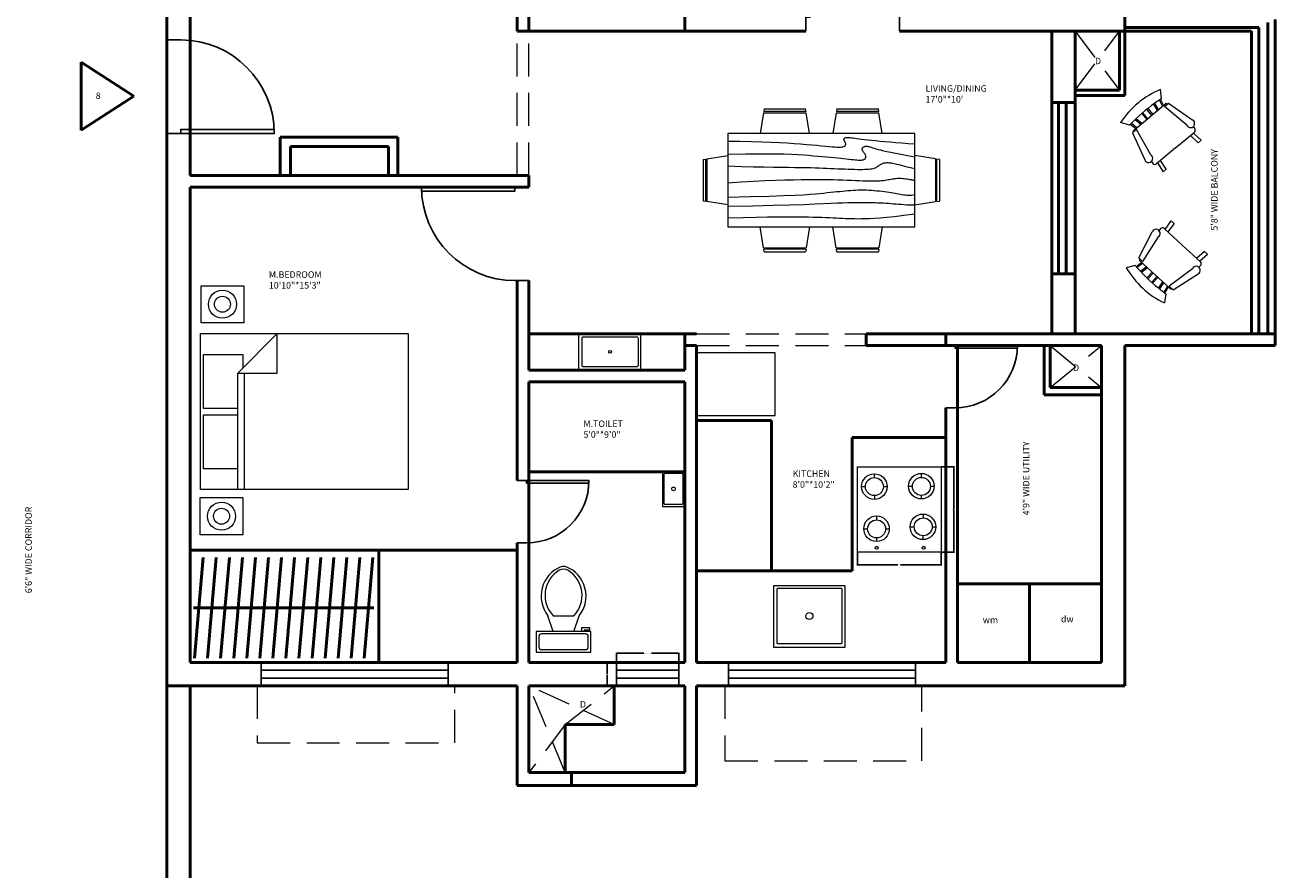
# Model space of a CAD drawing. Units: inches. Extents: x 291 to 2631, y 456 to 2623.
# Tile 12 of 22: x 2114 to 2595, y 1042 to 1367. Entities that reach past the tile are written whole.
import ezdxf

# ---------------------------------------------------------------- set-up
doc = ezdxf.new("R2010")
doc.units = ezdxf.units.IN
doc.linetypes.add('DASHED', pattern=[19.05, 12.7, -6.35])
for name, color, linetype, lineweight in [('A-ANNO-DIMS', 2, 'Continuous', 18), ('A-ANNO-TEXT', 3, 'Continuous', 25), ('A-AREA-IDEN', 7, 'Continuous', 25), ('A-DOOR', 3, 'Continuous', 25), ('A-EQPM', 8, 'Continuous', 18), ('A-FLOR-FIXT', 9, 'Continuous', 18), ('A-FLOR-OVHD', 1, 'DASHED', 18), ('A-FURN', 8, 'Continuous', 18), ('A-GLAZ', 4, 'Continuous', 25), ('A-WALL', 7, 'Continuous', 50)]:
    doc.layers.add(name, color=color, linetype=linetype, lineweight=lineweight)
doc.styles.get("Standard").update_dxf_attribs({"font": 'arial.ttf'})
doc.dimstyles.get("Standard").update_dxf_attribs({"dimtxt": 0.18, "dimasz": 0.18, "dimexe": 0.18, "dimexo": 0.0625, "dimgap": 0.09, "dimtad": 0, "dimtih": 1, "dimtoh": 1, "dimdec": 4, "dimzin": 0, "dimdsep": 46, "dimtxsty": 'Standard', "dimcen": 0.09, "dimadec": 0, "dimazin": 0, "dimtfac": 1, "dimtdec": 4, "dimtofl": 0, "dimtmove": 0, "dimatfit": 3, "dimfxl": 1, "dimtolj": 1, "dimtzin": 0, "dimarcsym": 0})

# ---------------------------------------------------------------- blocks, each defined once
blk = doc.blocks.new('*U2')
for p, q in [((0, 0), (0, -6)), ((40, 0), (40, -6))]:
    blk.add_line(p, q)
blk.add_lwpolyline([(0, 0), (0, 40), (1.75, 40), (1.75, 0)], close=True)
blk.add_arc((0, 0), 40, 0, 90)
blk = doc.blocks.new('Bed - Queen')
for p, q in [((0, -80.00003), (0, 0)), ((0, 0), (59.99999, 0)), ((59.99999, 0), (59.99999, -80.00003)), ((7.99999, -1.2), (28.79998, -1.2)), ((7.99999, -14.4), (7.99999, -1.2)), ((28.79998, -1.2), (28.79998, -14.4)), ((31.19999, -1.2), (51.99999, -1.2)), ((31.19999, -14.4), (31.19999, -1.2)), ((51.99999, -1.2), (51.99999, -16.4)), ((0, -14.4), (44.8, -14.4)), ((59.99999, -29.6), (44.8, -14.4)), ((44.8, -14.4), (44.8, -29.6)), ((44.8, -16.8), (0, -16.8)), ((51.99999, -16.4), (46.79936, -16.4)), ((44.8, -29.6), (59.99999, -29.6)), ((59.99999, -80.00003), (0, -80.00003))]:
    blk.add_line(p, q)
blk = doc.blocks.new('Toilet - top')
for p, q in [((9.5, -6), (9.5, -2)), ((-10, -8.5), (-8, -8.5)), ((-10, -9.5), (-10, -8.5)), ((-7, -9.5), (-10, -9.5)), ((-8, -8.5), (-8, -8)), ((-7, -8), (-7, -9.5)), ((-4, -8), (-6, -14)), ((4, -8), (6, -14)), ((4, -14), (-4, -14))]:
    blk.add_line(p, q)
blk.add_lwpolyline([(10.5, -8), (10.5, 0), (-10.5, 0), (-10.5, -8)], close=True)
for points in [[(-9.5, -2), (-9.5, -6)], [(8.5, -1), (-8.5, -1)], [(-8.5, -7), (8.5, -7)]]:
    blk.add_lwpolyline(points)
for centre, radius, start, end in [((-8.62, -1.88), 0.884, 81.8699, 188.1301), ((8.62, -1.88), 0.884, 351.8699, 98.1301), ((-8.62, -6.12), 0.884, 171.8699, 278.1301), ((8.62, -6.12), 0.884, 261.8699, 8.1301), ((3.52, -21.58), 12.17, 141.4691, 247.9714), ((4.2, -21.82), 11.33, 136.3677, 238.9468), ((-3.52, -21.58), 12.17, 292.0284, 38.5307), ((-4.2, -21.82), 11.33, 301.053, 43.6321), ((0, -27.88), 4, 245.7318, 294.2682), ((0, -29), 4, 254.8605, 285.1395)]:
    blk.add_arc(centre, radius, start, end)
blk = doc.blocks.new('Chair - Rocking')
for p, q in [((-8, -4.5), (-10, -1.5)), ((-7.5, -4.5), (-7, -7)), ((-6.5, -7), (-7.02225, -4.43)), ((-4.5, -7), (-4.96674, -4.19951)), ((-4, -7), (-4.40532, -4.16272)), ((-1.5, -4.05012), (-1.5, -7)), ((-1, -7), (-1, -4.05012)), ((1, -7), (1, -4.04655)), ((1.5, -4.05012), (1.5, -7)), ((4, -7), (4.40187, -4.18694)), ((4.5, -7), (4.96761, -4.19437)), ((6.5, -7), (7, -4.4057)), ((7.5, -4.5), (7, -7)), ((8, -4.5), (10, -1.5)), ((-9, -7.5), (-12, -18.49999)), ((-7, -7.5), (-9, -7.5)), ((-9, -18.49999), (-7, -7.5)), ((-8.23428, -6.99939), (-8.3093, -7.47958)), ((-8.23041, -7), (8.23915, -7)), ((7, -7.5), (9, -7.5)), ((9, -18.49999), (7, -7.5)), ((8.31071, -7.48854), (8.23449, -7.00073)), ((9, -7.5), (12, -18.49999)), ((-10.36644, -20.64523), (-10.5, -21.49999)), ((-9, -22.49999), (-9.5, -26.49999)), ((0, -22.49999), (-9.5, -22.49999)), ((-8, -26.49999), (-7.5, -22.49999)), ((0, -22.49999), (9.5, -22.49999)), ((8, -26.49999), (7.5, -22.49999)), ((9, -22.49999), (9.5, -26.49999)), ((10.5, -21.49999), (10.3575, -20.58798)), ((-9.5, -26.49999), (-8, -26.49999)), ((9.5, -26.49999), (8, -26.49999))]:
    blk.add_line(p, q)
for centre, radius, start, end in [((0, -34.08333), 34.08333, 72.93847, 107.0615), ((0, -68.25004), 64.25, 93.92211, 97.15267), ((0, -68.25004), 64.25, 82.84733, 93.92211), ((-10.5, -18.99999), 1.58114, 161.5651, 18.43495), ((10.5, -18.99999), 1.58114, 161.5651, 18.43495), ((-9.5, -21.49999), 1, 180, 270), ((9.5, -21.49999), 1, 270, 0)]:
    blk.add_arc(centre, radius, start, end)
blk = doc.blocks.new('Dining Set - 36 x 72 in.')
for p, q in [((-22.2343, 26.00059), (-23.4847, 17.99762)), ((-22.2304, 26), (-5.7608, 26)), ((-22, 27.5), (-22.1562, 26.50042)), ((-5.8416, 26.5), (-22.1534, 26.5)), ((-22, 27.5), (-6, 27.5)), ((-5.8437, 26.49966), (-6, 27.5)), ((-4.5152, 17.99762), (-5.7655, 25.99926)), ((5.7657, 26.00059), (4.5153, 17.99762)), ((5.7696, 26), (22.2392, 26)), ((6, 27.5), (5.8438, 26.50042)), ((22.1584, 26.5), (5.8466, 26.5)), ((6, 27.5), (22, 27.5)), ((22.1563, 26.49966), (22, 27.5)), ((23.4848, 17.99762), (22.2345, 25.99926)), ((36, 18), (-36, 18)), ((-36, 18), (-36, -18)), ((36, -18), (36, 18)), ((-45.5, 8), (-44.5004, 8.15617)), ((-45.5, 8), (-45.5, -8)), ((-44.5, -8.15843), (-44.5, 8.15338)), ((-44.0006, 8.23428), (-35.9976, 9.48474)), ((-44, 8.23041), (-44, -8.23915)), ((44.0006, 8.23428), (35.9976, 9.48474)), ((44, 8.23041), (44, -8.23915)), ((44.5, -8.15843), (44.5, 8.15338)), ((45.5, 8), (44.5005, 8.15617)), ((45.5, 8), (45.5, -8)), ((-44.4997, -8.15631), (-45.5, -8)), ((-35.9976, -9.48476), (-43.9993, -8.2345)), ((35.9976, -9.48476), (43.9993, -8.2345)), ((44.4997, -8.15631), (45.5, -8)), ((-36, -18), (36, -18)), ((-22.2343, -26.0006), (-23.4847, -17.99762)), ((-4.5152, -17.99762), (-5.7655, -25.99928)), ((5.7657, -26.0006), (4.5153, -17.99762)), ((23.4848, -17.99762), (22.2345, -25.99928)), ((-22.2304, -26), (-5.7608, -26)), ((-22, -27.5), (-22.1562, -26.50044)), ((-5.8416, -26.5), (-22.1534, -26.5)), ((-22, -27.5), (-6, -27.5)), ((-5.8437, -26.49967), (-6, -27.5)), ((5.7696, -26), (22.2392, -26)), ((6, -27.5), (5.8438, -26.50044)), ((22.1584, -26.5), (5.8466, -26.5)), ((6, -27.5), (22, -27.5)), ((22.1563, -26.49967), (22, -27.5))]:
    blk.add_line(p, q)
for points in [[(-36, 15), (-31.1772, 14.97754), (-26.8079, 14.91406), (-22.8538, 14.81543), (-19.276, 14.6875), (-16.0362, 14.53613), (-13.0957, 14.36718), (-10.4159, 14.18652), (-7.9583, 14), (-5.6904, 13.81315), (-3.6035, 13.63021), (-1.6954, 13.45508), (0.0365, 13.29166), (1.5945, 13.14388), (2.9811, 13.01562), (4.1988, 12.9108), (5.25, 12.83333), (6.1393, 12.78613), (6.8802, 12.76823), (7.4883, 12.77767), (7.9792, 12.8125), (8.3685, 12.87077), (8.6719, 12.95052), (8.9049, 13.0498), (9.0833, 13.16666), (9.2205, 13.29899), (9.3216, 13.44401), (9.3895, 13.59879), (9.4271, 13.76041), (9.4373, 13.92594), (9.4232, 14.09245), (9.3875, 14.257), (9.3333, 14.41666), (9.2638, 14.56917), (9.1836, 14.71484), (9.0975, 14.85465), (9.0104, 14.98958), (8.9272, 15.1206), (8.8529, 15.2487), (8.7922, 15.37483), (8.75, 15.5), (8.7305, 15.62467), (8.7344, 15.74739), (8.7617, 15.86621), (8.8125, 15.97916), (8.8867, 16.08431), (8.9844, 16.17968), (9.1055, 16.26334), (9.25, 16.33333), (9.4189, 16.38802), (9.6172, 16.42708), (9.8506, 16.45052), (10.125, 16.45833), (10.4463, 16.45052), (10.8203, 16.42708), (11.2529, 16.38802), (11.75, 16.33333), (12.3184, 16.26318), (12.9694, 16.17838), (13.7151, 16.07991), (14.5677, 15.96875), (15.5395, 15.84586), (16.6426, 15.71224), (17.8893, 15.56884), (19.2917, 15.41666), (20.859, 15.25667), (22.5879, 15.08984), (24.4721, 14.91715), (26.5052, 14.73958), (28.6809, 14.5581), (30.9929, 14.3737), (33.4347, 14.18733), (36, 14)], [(-36, 10), (-28.9766, 10.14274), (-23.1725, 10.20442), (-18.4241, 10.19775), (-14.5677, 10.13541), (-11.4399, 10.03011), (-8.877, 9.89453), (-6.7154, 9.74137), (-4.7917, 9.58333), (-2.9698, 9.43082), (-1.2246, 9.28515), (0.4415, 9.14534), (2.026, 9.01041), (3.5266, 8.87939), (4.9408, 8.7513), (6.266, 8.62516), (7.5, 8.5), (8.6411, 8.37549), (9.6914, 8.2539), (10.6538, 8.13818), (11.5312, 8.03125), (12.3267, 7.93603), (13.043, 7.85547), (13.6831, 7.79248), (14.25, 7.75), (14.7471, 7.7303), (15.1797, 7.73307), (15.5537, 7.75732), (15.875, 7.80208), (16.1494, 7.86637), (16.3828, 7.94922), (16.5811, 8.04964), (16.75, 8.16666), (16.8944, 8.29915), (17.0143, 8.44531), (17.1089, 8.60319), (17.1771, 8.77083), (17.218, 8.94629), (17.2305, 9.1276), (17.2137, 9.31282), (17.1667, 9.5), (17.0895, 9.6875), (16.987, 9.875), (16.8649, 10.0625), (16.7292, 10.25), (16.5856, 10.4375), (16.4401, 10.625), (16.2985, 10.8125), (16.1667, 11), (16.05, 11.18733), (15.9518, 11.3737), (15.8752, 11.5581), (15.8229, 11.73958), (15.798, 11.91715), (15.8034, 12.08984), (15.842, 12.25667), (15.9167, 12.41666), (16.0295, 12.56836), (16.1784, 12.70833), (16.3605, 12.83268), (16.5729, 12.9375), (16.8127, 13.01888), (17.0768, 13.07291), (17.3625, 13.0957), (17.6667, 13.08333), (17.9894, 13.03312), (18.3418, 12.94726), (18.7382, 12.82918), (19.1927, 12.68229), (19.7195, 12.51001), (20.3327, 12.31575), (21.0465, 12.10294), (21.875, 11.875), (22.8357, 11.63354), (23.959, 11.37304), (25.2786, 11.08618), (26.8282, 10.76562), (28.6414, 10.40405), (30.752, 9.99414), (33.1936, 9.52856), (36, 9)], [(-36, 5.5), (-30.7157, 5.3348), (-26.069, 5.20963), (-21.9946, 5.11767), (-18.4271, 5.05208), (-15.3009, 5.00602), (-12.5508, 4.97265), (-10.1112, 4.94515), (-7.9167, 4.91666), (-5.909, 4.88167), (-4.0586, 4.83984), (-2.3429, 4.79215), (-0.7396, 4.73958), (0.7739, 4.6831), (2.22, 4.6237), (3.6213, 4.56233), (5, 4.5), (6.373, 4.43782), (7.7344, 4.3776), (9.0723, 4.32129), (10.375, 4.27083), (11.6309, 4.22819), (12.8281, 4.19531), (13.9551, 4.17415), (15, 4.16666), (15.954, 4.17448), (16.819, 4.19791), (17.6001, 4.23698), (18.3021, 4.29166), (18.9299, 4.36198), (19.4883, 4.44791), (19.9823, 4.54948), (20.4167, 4.66666), (20.7969, 4.79899), (21.1302, 4.94401), (21.4245, 5.09879), (21.6875, 5.26041), (21.9271, 5.42594), (22.1511, 5.59245), (22.3672, 5.757), (22.5834, 5.91666), (22.8065, 6.06868), (23.0404, 6.21093), (23.2879, 6.34147), (23.5521, 6.45833), (23.8358, 6.55957), (24.142, 6.64323), (24.4735, 6.70735), (24.8334, 6.75), (25.2235, 6.76969), (25.642, 6.76692), (26.0858, 6.74267), (26.5521, 6.69791), (27.0379, 6.63362), (27.5404, 6.55078), (28.0565, 6.45036), (28.5834, 6.33333), (29.1242, 6.19987), (29.7071, 6.04687), (30.3661, 5.87044), (31.1354, 5.66666), (32.0493, 5.43164), (33.142, 5.16146), (34.4475, 4.85221), (36, 4.5)], [(-36, -1), (-30.7915, -0.6591), (-26.0195, -0.38216), (-21.6519, -0.16284), (-17.6563, 0.00521), (-14.0005, 0.12833), (-10.6523, 0.21289), (-7.5796, 0.26522), (-4.75, 0.29166), (-2.134, 0.29793), (0.2878, 0.28711), (2.5317, 0.26163), (4.6146, 0.22396), (6.5529, 0.17651), (8.3633, 0.12174), (10.0623, 0.06209), (11.6667, 0), (13.1899, -0.06201), (14.6341, -0.1211), (15.9982, -0.17432), (17.2813, -0.21875), (18.4823, -0.25147), (19.6003, -0.26953), (20.6343, -0.27002), (21.5834, -0.25), (22.4481, -0.20768), (23.2357, -0.14584), (23.9549, -0.06836), (24.6146, 0.02083), (25.2235, 0.11784), (25.7904, 0.21875), (26.3241, 0.31966), (26.8334, 0.41666), (27.3265, 0.50618), (27.8099, 0.58593), (28.2894, 0.65397), (28.7709, 0.70833), (29.2601, 0.74707), (29.763, 0.76823), (30.2855, 0.76985), (30.8334, 0.75), (31.4088, 0.70784), (31.9994, 0.64713), (32.589, 0.57275), (33.1615, 0.48958), (33.7008, 0.4025), (34.1908, 0.3164), (34.6153, 0.23616), (34.9584, 0.16666), (35.2099, 0.11165), (35.3848, 0.07031), (35.504, 0.04069), (35.5886, 0.02083), (35.6594, 0.00879), (35.7377, 0.0026), (35.8442, 0.00032), (36, 0)], [(-36, -6.5), (-27.1843, -6.31267), (-20.084, -6.1263), (-14.469, -5.9419), (-10.1094, -5.76042), (-6.7752, -5.58285), (-4.2363, -5.41016), (-2.2629, -5.24333), (-0.625, -5.08334), (0.8708, -4.93099), (2.2715, -4.78646), (3.5872, -4.64974), (4.8281, -4.52084), (6.0046, -4.39974), (7.127, -4.28646), (8.2053, -4.18099), (9.25, -4.08334), (10.2705, -3.99382), (11.2734, -3.91407), (12.2647, -3.84603), (13.25, -3.79167), (14.2354, -3.75293), (15.2266, -3.73177), (16.2295, -3.73015), (17.25, -3.75), (18.2912, -3.79248), (19.3451, -3.85547), (20.4009, -3.93604), (21.4479, -4.03125), (22.4754, -4.13819), (23.4727, -4.25391), (24.4289, -4.37549), (25.3334, -4.5), (26.1785, -4.62492), (26.9694, -4.74935), (27.7145, -4.87281), (28.4219, -4.99479), (29.1, -5.11483), (29.7572, -5.23242), (30.4016, -5.34709), (31.0417, -5.45834), (31.6837, -5.56437), (32.3262, -5.65821), (32.9658, -5.73153), (33.599, -5.77604), (34.2224, -5.78345), (34.8327, -5.74545), (35.4264, -5.65373), (36, -5.5)], [(-36, -10), (-26.4022, -9.81299), (-18.4675, -9.62891), (-11.9839, -9.45069), (-6.7396, -9.28125), (-2.5226, -9.12354), (0.8789, -8.98047), (3.6769, -8.85498), (6.0833, -8.75), (8.2767, -8.66765), (10.3021, -8.60677), (12.1712, -8.56543), (13.8958, -8.54167), (15.4876, -8.53353), (16.9583, -8.53907), (18.3197, -8.55632), (19.5834, -8.58334), (20.7616, -8.61841), (21.8685, -8.66081), (22.9188, -8.71004), (23.9271, -8.76563), (24.9081, -8.82707), (25.8763, -8.89388), (26.8465, -8.96558), (27.8334, -9.04167), (28.8474, -9.12118), (29.8828, -9.20117), (30.93, -9.27824), (31.9792, -9.34896), (33.0205, -9.40991), (34.0443, -9.45768), (35.0407, -9.48885), (36, -9.5)], [(-36, -14.5), (-30.0881, -14.33513), (-25.0332, -14.21224), (-20.7312, -14.12647), (-17.0781, -14.07292), (-13.97, -14.04671), (-11.3027, -14.04297), (-8.9724, -14.05681), (-6.875, -14.08334), (-4.9224, -14.11833), (-3.0905, -14.16016), (-1.3709, -14.20785), (0.2448, -14.26042), (1.7647, -14.3169), (3.1973, -14.3763), (4.5507, -14.43767), (5.8333, -14.5), (7.0554, -14.5621), (8.235, -14.62175), (9.3922, -14.67652), (10.5469, -14.72396), (11.7192, -14.76164), (12.929, -14.78711), (14.1965, -14.79794), (15.5417, -14.79167), (16.9933, -14.76424), (18.6152, -14.70508), (20.4804, -14.60197), (22.6615, -14.44271), (25.2312, -14.21509), (28.2624, -13.9069), (31.8277, -13.50594), (36, -13)]]:
    blk.add_lwpolyline(points)
blk = doc.blocks.new('WIN-1800')
for p, q in [((0, 9), (72, 9)), ((0, 0), (0, 9)), ((0, 6), (72, 6)), ((72, 9), (72, 0)), ((72, 3), (0, 3)), ((72, 0), (0, 0))]:
    blk.add_line(p, q)
blk = doc.blocks.new('COOKTOP')
for p, q in [((6.54, 28.68), (6.54, 30.14)), ((24.62, 30.31), (24.62, 28.76)), ((1.62, 25.22), (3.08, 25.22)), ((10, 25.22), (11.46, 25.22)), ((19.7, 25.39), (21.21, 25.39)), ((28.13, 25.39), (29.54, 25.39)), ((6.54, 21.76), (6.54, 20.3)), ((24.62, 21.83), (24.62, 20.47)), ((25.35, 14.65), (25.34, 13.21)), ((7.38, 13.92), (7.38, 12.38)), ((20.32, 9.73), (21.89, 9.73)), ((28.81, 9.73), (30.16, 9.73)), ((2.46, 9), (3.95, 9)), ((7.38, 5.46), (7.38, 4.08)), ((10.87, 9), (12.3, 9)), ((25.26, 6.28), (25.24, 4.81))]:
    blk.add_line(p, q)
blk.add_lwpolyline([(0, 32.79), (32.25, 32.79), (32.25, 0), (0, 0)], close=True)
for centre, radius in [((6.54, 25.22), 4.92), ((24.62, 25.39), 4.92), ((6.54, 25.22), 3.46), ((24.67, 25.29), 3.46), ((25.24, 9.73), 4.92), ((7.38, 9), 4.92), ((7.41, 8.92), 3.46), ((25.35, 9.74), 3.46), ((7.38, 1.69), 0.572), ((25.5, 1.69), 0.572)]:
    blk.add_circle(centre, radius)
blk = doc.blocks.new('WIN-600')
for p, q in [((24, 9), (0, 9)), ((0, 9), (0, 0)), ((24, 6), (0, 6)), ((24, 0), (24, 9)), ((0, 3), (24, 3)), ((0, 0), (24, 0))]:
    blk.add_line(p, q)
blk = doc.blocks.new('*D26')
at = {"layer": 'A-ANNO-DIMS', "color": 0, "lineweight": -2, "transparency": 16777216}
for p, q in [((2341.38, 1121.58), (2341.38, 1125.3)), ((2341.56, 1125.12), (2351.9, 1125.12)), ((2365.2, 1125.12), (2354.86, 1125.12)), ((2365.38, 1121.58), (2365.38, 1125.3))]:
    blk.add_line(p, q, dxfattribs=at)
at = {"layer": 'A-ANNO-DIMS', "color": 0, "transparency": 16777216}
for points in [[(2341.56, 1125.15), (2341.56, 1125.09), (2341.38, 1125.12)], [(2365.2, 1125.15), (2365.2, 1125.09), (2365.38, 1125.12)]]:
    blk.add_solid(points, dxfattribs=at)
at = {"layer": 'DEFPOINTS', "color": 0, "transparency": 16777216}
for p in [(2341.38, 1125.12), (2341.38, 1121.52), (2365.38, 1121.52)]:
    blk.add_point(p, dxfattribs=at)
at = {"layer": 'A-ANNO-DIMS', "color": 0, "transparency": 16777216, "insert": (2353.38, 1125.12), "char_height": 0.18, "attachment_point": 5}
blk.add_mtext('\\A1;WINDOW W600 24 TYP.', dxfattribs=at)
blk = doc.blocks.new('*D27')
at = {"layer": 'A-ANNO-DIMS', "color": 0, "lineweight": -2, "transparency": 16777216}
for p, q in [((2341.32, 1121.52), (2337.6, 1121.52)), ((2337.78, 1121.34), (2337.78, 1117.2)), ((2341.32, 1112.52), (2337.6, 1112.52)), ((2337.78, 1112.7), (2337.78, 1116.83))]:
    blk.add_line(p, q, dxfattribs=at)
at = {"layer": 'A-ANNO-DIMS', "color": 0, "transparency": 16777216}
for points in [[(2337.75, 1121.34), (2337.81, 1121.34), (2337.78, 1121.52)], [(2337.75, 1112.7), (2337.81, 1112.7), (2337.78, 1112.52)]]:
    blk.add_solid(points, dxfattribs=at)
at = {"layer": 'DEFPOINTS', "color": 0, "transparency": 16777216}
for p in [(2341.38, 1121.52), (2337.78, 1112.52), (2341.38, 1112.52)]:
    blk.add_point(p, dxfattribs=at)
at = {"layer": 'A-ANNO-DIMS', "color": 0, "transparency": 16777216, "insert": (2337.78, 1117.02), "char_height": 0.18, "attachment_point": 5}
blk.add_mtext('\\A1;9 TYP.', dxfattribs=at)
blk = doc.blocks.new('*D44')
at = {"layer": 'A-ANNO-DIMS', "color": 0, "lineweight": -2, "transparency": 16777216}
for p, q in [((2466.51, 1196.81), (2471.55, 1196.81)), ((2471.37, 1196.63), (2471.37, 1180.59)), ((2471.37, 1164.19), (2471.37, 1180.23)), ((2466.51, 1164.01), (2471.55, 1164.01))]:
    blk.add_line(p, q, dxfattribs=at)
at = {"layer": 'A-ANNO-DIMS', "color": 0, "transparency": 16777216}
for points in [[(2471.34, 1196.63), (2471.4, 1196.63), (2471.37, 1196.81)], [(2471.34, 1164.19), (2471.4, 1164.19), (2471.37, 1164.01)]]:
    blk.add_solid(points, dxfattribs=at)
at = {"layer": 'DEFPOINTS', "color": 0, "transparency": 16777216}
for p in [(2466.45, 1196.81), (2471.37, 1196.81), (2466.45, 1164.01)]:
    blk.add_point(p, dxfattribs=at)
at = {"layer": 'A-ANNO-DIMS', "color": 0, "transparency": 16777216, "insert": (2471.37, 1180.41), "char_height": 0.18, "attachment_point": 5}
blk.add_mtext('\\A1;COOKTOP 33 TYP.', dxfattribs=at)
blk = doc.blocks.new('*D45')
at = {"layer": 'A-ANNO-DIMS', "color": 0, "lineweight": -2, "transparency": 16777216}
for p, q in [((2434.2, 1163.95), (2434.2, 1158.91)), ((2466.45, 1163.95), (2466.45, 1158.91)), ((2434.38, 1159.09), (2449.8, 1159.09)), ((2466.27, 1159.09), (2450.85, 1159.09))]:
    blk.add_line(p, q, dxfattribs=at)
at = {"layer": 'A-ANNO-DIMS', "color": 0, "transparency": 16777216}
for points in [[(2434.38, 1159.12), (2434.38, 1159.06), (2434.2, 1159.09)], [(2466.27, 1159.12), (2466.27, 1159.06), (2466.45, 1159.09)]]:
    blk.add_solid(points, dxfattribs=at)
at = {"layer": 'DEFPOINTS', "color": 0, "transparency": 16777216}
for p in [(2434.2, 1164.01), (2466.45, 1164.01), (2466.45, 1159.09)]:
    blk.add_point(p, dxfattribs=at)
at = {"layer": 'A-ANNO-DIMS', "color": 0, "transparency": 16777216, "insert": (2450.32, 1159.09), "char_height": 0.18, "attachment_point": 5}
blk.add_mtext('\\A1;32 TYP.', dxfattribs=at)

msp = doc.modelspace()

# ---------------------------------------------------------------- linework, layer by layer
at = {"layer": 'A-FLOR-OVHD'}
for p, q in [((2303.21, 1309.02), (2303.21, 1364.52)), ((2307.71, 1309.02), (2307.71, 1364.52)), ((2518.05, 1364.52), (2535.11, 1341.75)), ((2518.05, 1341.75), (2535.11, 1364.52)), ((2372.21, 1248.02), (2437.63, 1248.02)), ((2372.21, 1243.52), (2437.63, 1243.52)), ((2508.4, 1243.52), (2528.21, 1227.33)), ((2508.4, 1227.33), (2528.21, 1243.52)), ((2203.04, 1112.52), (2203.04, 1090.62)), ((2279.1, 1090.62), (2279.1, 1112.52)), ((2321.68, 1079.22), (2307.71, 1112.52)), ((2340.52, 1097.69), (2307.71, 1112.52)), ((2321.68, 1097.69), (2340.52, 1112.52)), ((2383.18, 1112.52), (2383.18, 1083.64)), ((2458.99, 1083.64), (2458.99, 1112.52)), ((2321.68, 1097.69), (2307.71, 1079.22)), ((2203.04, 1090.62), (2279.1, 1090.62)), ((2383.18, 1083.64), (2458.99, 1083.64))]:
    msp.add_line(p, q, dxfattribs=at)
at = {"layer": 'A-FURN'}
for points in [[(2181.41, 1266.56), (2197.89, 1266.56), (2197.89, 1252.27), (2181.41, 1252.27)], [(2326.89, 1248.02), (2350.7, 1248.02), (2350.7, 1234.02), (2326.89, 1234.02)], [(2372.21, 1216.65), (2402.55, 1216.65), (2402.55, 1240.71), (2372.21, 1240.71)], [(2367.71, 1194.96), (2359.18, 1194.96), (2359.18, 1181.59), (2367.71, 1181.59)], [(2181.05, 1184.99), (2197.53, 1184.99), (2197.53, 1170.69), (2181.05, 1170.69)], [(2401.96, 1151.2), (2429.39, 1151.2), (2429.39, 1127.3), (2401.96, 1127.3)]]:
    msp.add_lwpolyline(points, close=True, dxfattribs=at)
for points in [[(2328.66, 1246.87), (2349.21, 1246.87, -0.414214), (2349.71, 1246.37), (2349.71, 1235.77, -0.414214), (2349.21, 1235.27), (2328.66, 1235.27, -0.414214), (2328.16, 1235.77), (2328.16, 1246.37, -0.414214)], [(2360.23, 1194.35), (2366.48, 1194.35, -0.414214), (2366.98, 1193.85), (2366.98, 1182.82, -0.414214), (2366.48, 1182.32), (2360.23, 1182.32, -0.414214), (2359.73, 1182.82), (2359.73, 1193.85, -0.414214)], [(2403.59, 1150.09), (2427.89, 1150.09, -0.414214), (2428.19, 1149.79), (2428.19, 1129.02, -0.414214), (2427.89, 1128.72), (2403.59, 1128.72, -0.414214), (2403.29, 1129.02), (2403.29, 1149.79, -0.414214)]]:
    msp.add_lwpolyline(points, format="xyb", close=True, dxfattribs=at)
for centre, radius in [((2189.65, 1259.42), 5.39), ((2189.65, 1259.42), 3.08), ((2338.93, 1241.07), 0.547), ((2363.35, 1188.34), 0.716), ((2189.29, 1177.84), 5.39), ((2189.29, 1177.84), 3.08), ((2415.74, 1139.4), 1.36)]:
    msp.add_circle(centre, radius, dxfattribs=at)
at = {"layer": 'A-WALL'}
for p, q in [((2168.21, 1650.64), (2168.21, 1112.52)), ((2537.21, 1498.02), (2537.21, 1364.52)), ((2177.21, 1489.02), (2177.21, 1309.02)), ((2303.21, 1489.02), (2303.21, 1364.52)), ((2307.71, 1382.52), (2307.71, 1364.52)), ((2367.71, 1382.52), (2367.71, 1364.52)), ((2592.31, 1367.87), (2592.31, 1248.02)), ((2595.05, 1369.02), (2595.05, 1364.52)), ((2367.71, 1364.52), (2303.21, 1364.52)), ((2367.71, 1364.52), (2414.38, 1364.52)), ((2450.38, 1364.52), (2537.21, 1364.52)), ((2509.05, 1364.52), (2509.05, 1248.02)), ((2518.05, 1364.52), (2518.05, 1248.02)), ((2535.11, 1341.75), (2535.11, 1364.52)), ((2537.21, 1365.96), (2588.84, 1365.96)), ((2537.21, 1364.52), (2586.05, 1364.52)), ((2537.21, 1339.74), (2537.21, 1364.52)), ((2586.05, 1364.52), (2586.05, 1248.02)), ((2588.84, 1365.96), (2588.84, 1248.02)), ((2595.05, 1364.52), (2595.05, 1248.02)), ((2135.28, 1352.63), (2135.28, 1326.38)), ((2135.28, 1352.63), (2155.56, 1339.52)), ((2155.56, 1339.52), (2135.28, 1326.38)), ((2518.05, 1341.75), (2535.11, 1341.75)), ((2518.05, 1339.74), (2537.21, 1339.74)), ((2509.05, 1337.11), (2518.05, 1337.11)), ((2511.67, 1337.11), (2511.67, 1271.15)), ((2514.63, 1337.09), (2514.63, 1271.15)), ((2211.92, 1309.02), (2211.92, 1323.75)), ((2211.92, 1323.75), (2257.17, 1323.75)), ((2215.8, 1308.96), (2215.8, 1320.14)), ((2215.8, 1320.14), (2253.6, 1320.14)), ((2253.6, 1320.14), (2253.6, 1309.02)), ((2257.17, 1323.75), (2257.17, 1309.02)), ((2177.21, 1309.02), (2307.71, 1309.02)), ((2307.71, 1309.02), (2307.71, 1304.52)), ((2177.21, 1304.52), (2307.71, 1304.52)), ((2177.21, 1304.52), (2177.21, 1121.52)), ((2509.05, 1271.15), (2518.05, 1271.15)), ((2303.21, 1268.52), (2303.21, 1191.55)), ((2307.71, 1268.52), (2307.71, 1234.02)), ((2307.71, 1248.02), (2372.21, 1248.02)), ((2367.71, 1248.02), (2367.71, 1234.02)), ((2437.63, 1248.02), (2437.63, 1243.52)), ((2437.63, 1248.02), (2537.21, 1248.02)), ((2468.21, 1248.02), (2468.21, 1243.52)), ((2537.21, 1248.02), (2595.05, 1248.02)), ((2595.05, 1243.52), (2595.05, 1248.02)), ((2367.71, 1243.52), (2372.21, 1243.52)), ((2372.21, 1243.52), (2372.21, 1121.52)), ((2437.63, 1243.52), (2528.21, 1243.52)), ((2472.71, 1243.52), (2472.71, 1121.52)), ((2506.09, 1243.52), (2506.09, 1224.56)), ((2508.4, 1243.52), (2508.4, 1227.33)), ((2528.21, 1243.52), (2528.21, 1121.52)), ((2537.21, 1243.52), (2537.21, 1112.52)), ((2537.21, 1243.52), (2595.05, 1243.52)), ((2307.71, 1234.02), (2367.71, 1234.02)), ((2307.71, 1229.52), (2367.71, 1229.52)), ((2307.71, 1229.52), (2307.71, 1194.96)), ((2367.71, 1229.52), (2367.71, 1121.52)), ((2506.09, 1224.56), (2528.21, 1224.56)), ((2508.4, 1227.33), (2528.21, 1227.33)), ((2468.21, 1219.52), (2468.21, 1121.52)), ((2372.21, 1214.62), (2401.16, 1214.62)), ((2401.16, 1214.62), (2401.16, 1156.78)), ((2432.14, 1156.78), (2432.14, 1208.18)), ((2432.14, 1208.18), (2468.21, 1208.18)), ((2307.71, 1194.96), (2367.71, 1194.96)), ((2307.71, 1194.96), (2307.71, 1121.52)), ((2303.21, 1167.55), (2303.21, 1121.52)), ((2177.21, 1164.75), (2303.21, 1164.75)), ((2178.89, 1123.13), (2182.26, 1161.91)), ((2183.92, 1123.13), (2187.29, 1161.91)), ((2188.95, 1123.13), (2192.32, 1161.91)), ((2193.98, 1123.13), (2197.35, 1161.91)), ((2199.01, 1123.13), (2202.38, 1161.91)), ((2204.04, 1123.13), (2207.4, 1161.91)), ((2209.06, 1123.13), (2212.43, 1161.91)), ((2214.09, 1123.13), (2217.46, 1161.91)), ((2219.12, 1123.13), (2222.49, 1161.91)), ((2224.15, 1123.13), (2227.52, 1161.91)), ((2229.18, 1123.13), (2232.55, 1161.91)), ((2234.21, 1123.13), (2237.57, 1161.91)), ((2239.24, 1123.13), (2242.6, 1161.91)), ((2244.26, 1123.13), (2247.63, 1161.91)), ((2249.83, 1164.75), (2249.83, 1121.52)), ((2401.16, 1156.78), (2372.21, 1156.78)), ((2401.16, 1156.78), (2432.14, 1156.78)), ((2472.71, 1151.84), (2528.21, 1151.84)), ((2500.46, 1151.84), (2500.46, 1121.52)), ((2178.53, 1142.52), (2247.92, 1142.52)), ((2177.21, 1121.52), (2303.21, 1121.52)), ((2307.71, 1121.52), (2367.71, 1121.52)), ((2372.21, 1121.52), (2468.21, 1121.52)), ((2472.71, 1121.52), (2528.21, 1121.52)), ((2168.21, 1112.52), (2303.21, 1112.52)), ((2168.21, 1112.52), (2168.21, 930.98)), ((2177.21, 1112.52), (2177.21, 930.98)), ((2303.21, 1112.52), (2303.21, 1074.13)), ((2307.71, 1112.52), (2307.71, 1079.22)), ((2307.71, 1112.52), (2367.71, 1112.52)), ((2340.52, 1097.69), (2340.52, 1112.52)), ((2367.71, 1079.22), (2367.71, 1112.52)), ((2372.21, 1112.52), (2372.21, 1079.22)), ((2372.21, 1112.52), (2537.21, 1112.52)), ((2321.68, 1079.22), (2321.68, 1097.69)), ((2321.68, 1097.69), (2340.52, 1097.69)), ((2307.71, 1079.22), (2367.71, 1079.22)), ((2324.1, 1079.22), (2324.1, 1074.13)), ((2372.21, 1079.22), (2372.21, 1074.13)), ((2303.21, 1074.13), (2372.21, 1074.13))]:
    msp.add_line(p, q, dxfattribs=at)

# ---------------------------------------------------------------- block references
at = {"layer": 'A-DOOR', "xscale": 0.9, "yscale": 0.9, "zscale": 0.9}
msp.add_blockref('*U2', (2414.38, 1369.92), dxfattribs=at)
at = {"layer": 'A-DOOR'}
for p, xscale, yscale, zscale, rotation in [((2173.61, 1325.13), -0.9, 0.9, 0.9, 270), ((2302.31, 1304.52), -0.9, 0.9, 0.9, 90), ((2471.81, 1243.52), 0.6, 0.6, 0.6, 270), ((2306.81, 1191.55), 0.6, 0.6, 0.6, 270)]:
    msp.add_blockref('*U2', p, dxfattribs=dict(at, xscale=xscale, yscale=yscale, zscale=zscale, rotation=rotation))
at = {"layer": 'A-EQPM'}
msp.add_blockref('COOKTOP', (2434.2, 1164.01), dxfattribs=at)
at = {"layer": 'A-FLOR-FIXT', "rotation": 180}
msp.add_blockref('Toilet - top', (2321.03, 1125.51), dxfattribs=at)
at = {"layer": 'A-FURN'}
for name, p, rotation in [('Chair - Rocking', (2542.3, 1336.86), 39.75679378516137), ('Chair - Rocking', (2544.08, 1265.6), 137.3178093086548), ('Bed - Queen', (2181.16, 1188.11), 90)]:
    msp.add_blockref(name, p, dxfattribs=dict(at, rotation=rotation))
msp.add_blockref('Dining Set - 36 x 72 in.', (2420.27, 1307.15), dxfattribs=at)
at = {"layer": 'A-GLAZ'}
for p in [(2204.58, 1112.52), (2384.58, 1112.52)]:
    msp.add_blockref('WIN-1800', p, dxfattribs=at)
at = {"layer": 'A-GLAZ', "rotation": 180}
msp.add_blockref('WIN-600', (2365.38, 1121.52), dxfattribs=at)

# ---------------------------------------------------------------- texts
at = {"layer": 'A-ANNO-TEXT', "char_height": 2.5, "attachment_point": 1}
for s, width, insert in [('D', 2.2604, (2525.7, 1354.3)), ('8', 7.2205, (2140.83, 1340.92)), ('D', 1.9791, (2517.27, 1236.26)), ('wm', 19.4631, (2482.5, 1139.16)), ('dw', 15.092, (2512.61, 1139.5)), ('D', 2.0493, (2327.31, 1106.7))]:
    msp.add_mtext_dynamic_manual_height_columns(s, width=width, gutter_width=12.5, heights=[0], dxfattribs=dict(at, insert=insert))
at = {"layer": 'A-AREA-IDEN', "char_height": 2.5, "attachment_point": 1}
for s, width, insert in [('LIVING/DINING\\P17\'0"*10\'', 56.5459, (2460.43, 1343.7)), ('M.BEDROOM\\P10\'10"*15\'3"', 59.2019, (2207.53, 1272.1)), ('M.TOILET\\P5\'0"*9\'0"', 47.3215, (2328.69, 1214.68)), ('KITCHEN\\P8\'0"*10\'2"', 27.0489, (2409.27, 1195.45))]:
    msp.add_mtext_dynamic_manual_height_columns(s, width=width, gutter_width=12.5, heights=[0], dxfattribs=dict(at, insert=insert))
at = {"layer": 'A-AREA-IDEN', "char_height": 2.5, "attachment_point": 1, "rotation": 90}
for s, width, insert in [('5\'8" WIDE BALCONY', 47.6459, (2570.44, 1287.76)), ('4\'9" WIDE UTILITY', 43.0323, (2497.93, 1178.17)), ('6\'6" WIDE CORRIDOR', 73.1508, (2113.73, 1148.18))]:
    msp.add_mtext_dynamic_manual_height_columns(s, width=width, gutter_width=12.5, heights=[0], dxfattribs=dict(at, insert=insert))

# ---------------------------------------------------------------- dimensions: what is measured, and where the dimension line sits
at = {"layer": 'A-ANNO-DIMS'}
for base, p1, p2, angle, text, picture, middle in [((2471.37, 1196.81), (2466.45, 1164.01), (2466.45, 1196.81), 90, 'COOKTOP <> TYP.', '*D44', (2471.37, 1180.41)), ((2341.38, 1125.12), (2365.38, 1121.52), (2341.38, 1121.52), 180, 'WINDOW W600 <> TYP.', '*D26', (2353.38, 1125.12)), ((2337.78, 1112.52), (2341.38, 1121.52), (2341.38, 1112.52), 270, '<> TYP.', '*D27', (2337.78, 1117.02))]:
    dim = msp.add_linear_dim(base=base, p1=p1, p2=p2, angle=angle, text=text, dimstyle='Standard', override={"dimdec": 0, "dimlfac": 1, "dimrnd": 0, "dimzin": 0, "dimdsep": 46, "dimlunit": 2}, dxfattribs=at)
    dim.commit()
    dim.dimension.update_dxf_attribs({"geometry": picture, "text_midpoint": middle})
dim = msp.add_linear_dim(base=(2466.45, 1159.09), p1=(2434.2, 1164.01), p2=(2466.45, 1164.01), text='<> TYP.', dimstyle='Standard', override={"dimdec": 0, "dimlfac": 1, "dimrnd": 0, "dimzin": 0, "dimdsep": 46, "dimlunit": 2}, dxfattribs=at)
dim.commit()
dim.dimension.update_dxf_attribs({"geometry": '*D45', "text_midpoint": (2450.32, 1159.09)})

doc.saveas('drawing.dxf')
